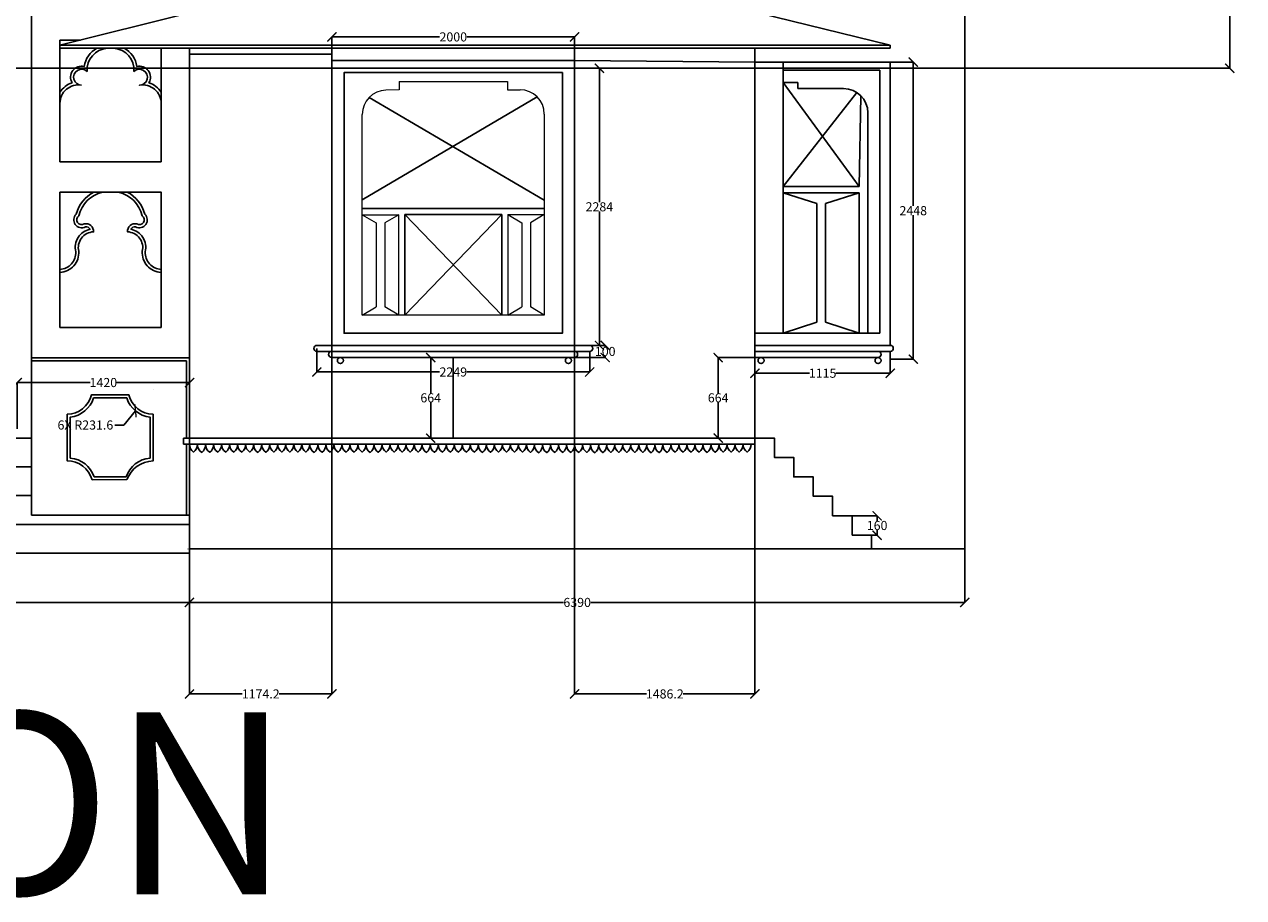
# Model space of a CAD drawing. Units: inches. Extents: x 829 to 33356404, y 1874 to 16983.
# Tile 8 of 9: x 16199 to 26248, y 1874 to 9069. Entities that reach past the tile are written whole.
import ezdxf

# ---------------------------------------------------------------- set-up
doc = ezdxf.new("R2010")
doc.units = ezdxf.units.IN
doc.header["$MEASUREMENT"] = 0
doc.header["$PDMODE"] = 3
for name, color, linetype, lineweight in [('A-ANNO-DIMS', 2, 'Continuous', 18), ('A-ANNO-TEXT', 7, 'Continuous', 25), ('A-ELEV', 7, 'Continuous', 25), ('A-GLAZ', 4, 'Continuous', 18)]:
    doc.layers.add(name, color=color, linetype=linetype, lineweight=lineweight)
doc.styles.get("Standard").update_dxf_attribs({"font": 'arial.ttf'})
doc.dimstyles.get("Standard").update_dxf_attribs({"dimtxt": 75, "dimasz": 75, "dimexe": 0.18, "dimexo": 0.0625, "dimgap": 0.09, "dimtad": 0, "dimtih": 1, "dimtoh": 1, "dimdec": 0, "dimzin": 0, "dimdsep": 46, "dimtxsty": 'Standard', "dimblk": 'ARCHTICK', "dimcen": 0.09, "dimadec": 0, "dimazin": 0, "dimtfac": 1, "dimtdec": 0, "dimtofl": 0, "dimtmove": 0, "dimatfit": 3, "dimfxl": 1, "dimtolj": 1, "dimtzin": 0, "dimarcsym": 0})

# ---------------------------------------------------------------- blocks, each defined once
blk = doc.blocks.new('_ArchTick')
at = {"color": 0, "linetype": 'ByBlock', "const_width": 0.15}
blk.add_lwpolyline([(-0.5, -0.5), (0.5, 0.5)], dxfattribs=at)
blk = doc.blocks.new('*D3')
at = {"layer": 'A-ANNO-DIMS', "color": 0, "lineweight": -2, "transparency": 16777216}
for p, q in [((9560, 4746), (9560, 4306)), ((17560, 4746), (17560, 4306)), ((9560, 4306), (13448, 4306)), ((17560, 4306), (13672, 4306))]:
    blk.add_line(p, q, dxfattribs=at)
at = {"layer": 'Defpoints', "color": 0, "transparency": 16777216}
for p in [(9560, 4746), (17560, 4746), (17560, 4306)]:
    blk.add_point(p, dxfattribs=at)
at = {"layer": 'A-ANNO-DIMS', "color": 0, "lineweight": -2, "transparency": 16777216, "xscale": 75, "yscale": 75, "zscale": 75, "rotation": 180}
blk.add_blockref('_ArchTick', (9560, 4306), dxfattribs=at)
at = {"layer": 'A-ANNO-DIMS', "color": 0, "lineweight": -2, "transparency": 16777216, "xscale": 75, "yscale": 75, "zscale": 75}
blk.add_blockref('_ArchTick', (17560, 4306), dxfattribs=at)
at = {"layer": 'A-ANNO-DIMS', "color": 0, "transparency": 16777216, "insert": (13560, 4306), "char_height": 75, "attachment_point": 5}
blk.add_mtext('\\A1;8000', dxfattribs=at)
blk = doc.blocks.new('*D4')
at = {"layer": 'A-ANNO-DIMS', "color": 0, "lineweight": -2, "transparency": 16777216}
for p, q in [((17560, 4746), (17560, 4306)), ((23950, 4746), (23950, 4306)), ((17560, 4306), (20643, 4306)), ((23950, 4306), (20867, 4306))]:
    blk.add_line(p, q, dxfattribs=at)
at = {"layer": 'Defpoints', "color": 0, "transparency": 16777216}
for p in [(17560, 4746), (23950, 4746), (23950, 4306)]:
    blk.add_point(p, dxfattribs=at)
at = {"layer": 'A-ANNO-DIMS', "color": 0, "lineweight": -2, "transparency": 16777216, "xscale": 75, "yscale": 75, "zscale": 75, "rotation": 180}
blk.add_blockref('_ArchTick', (17560, 4306), dxfattribs=at)
at = {"layer": 'A-ANNO-DIMS', "color": 0, "lineweight": -2, "transparency": 16777216, "xscale": 75, "yscale": 75, "zscale": 75}
blk.add_blockref('_ArchTick', (23950, 4306), dxfattribs=at)
at = {"layer": 'A-ANNO-DIMS', "color": 0, "transparency": 16777216, "insert": (20755, 4306), "char_height": 75, "attachment_point": 5}
blk.add_mtext('\\A1;6390', dxfattribs=at)
blk = doc.blocks.new('*D10')
at = {"layer": 'A-ANNO-DIMS', "color": 0, "lineweight": -2, "transparency": 16777216}
for p, q in [((19734, 6324), (19548, 6324)), ((19548, 6324), (19548, 6031)), ((19548, 5660), (19548, 5954)), ((19734, 5660), (19548, 5660))]:
    blk.add_line(p, q, dxfattribs=at)
at = {"layer": 'Defpoints', "color": 0, "transparency": 16777216}
for p in [(19548, 6324), (19734, 6324), (19734, 5660)]:
    blk.add_point(p, dxfattribs=at)
at = {"layer": 'A-ANNO-DIMS', "color": 0, "lineweight": -2, "transparency": 16777216, "xscale": 75, "yscale": 75, "zscale": 75}
for p, rotation in [((19548, 6324), 90), ((19548, 5660), 270)]:
    blk.add_blockref('_ArchTick', p, dxfattribs=dict(at, rotation=rotation))
at = {"layer": 'A-ANNO-DIMS', "color": 0, "transparency": 16777216, "insert": (19548, 5992), "char_height": 75, "attachment_point": 5}
blk.add_mtext('\\A1;664', dxfattribs=at)
blk = doc.blocks.new('*D11')
at = {"layer": 'A-ANNO-DIMS', "color": 0, "lineweight": -2, "transparency": 16777216}
for p, q in [((22220, 6324), (21916, 6324)), ((21917, 6324), (21917, 6031)), ((21917, 5660), (21917, 5954)), ((22220, 5660), (21916, 5660))]:
    blk.add_line(p, q, dxfattribs=at)
at = {"layer": 'Defpoints', "color": 0, "transparency": 16777216}
for p in [(21917, 6324), (22220, 6324), (22220, 5660)]:
    blk.add_point(p, dxfattribs=at)
at = {"layer": 'A-ANNO-DIMS', "color": 0, "lineweight": -2, "transparency": 16777216, "xscale": 75, "yscale": 75, "zscale": 75}
for p, rotation in [((21917, 6324), 90), ((21917, 5660), 270)]:
    blk.add_blockref('_ArchTick', p, dxfattribs=dict(at, rotation=rotation))
at = {"layer": 'A-ANNO-DIMS', "color": 0, "transparency": 16777216, "insert": (21917, 5992), "char_height": 75, "attachment_point": 5}
blk.add_mtext('\\A1;664', dxfattribs=at)
blk = doc.blocks.new('*D12')
at = {"layer": 'A-ANNO-DIMS', "color": 0, "lineweight": -2, "transparency": 16777216}
for p, q in [((23335, 6374), (23335, 6195)), ((22220, 6310), (22220, 6195)), ((22220, 6195), (22669, 6195)), ((23335, 6195), (22887, 6195))]:
    blk.add_line(p, q, dxfattribs=at)
at = {"layer": 'Defpoints', "color": 0, "transparency": 16777216}
for p in [(23335, 6374), (22220, 6310), (23335, 6195)]:
    blk.add_point(p, dxfattribs=at)
at = {"layer": 'A-ANNO-DIMS', "color": 0, "lineweight": -2, "transparency": 16777216, "xscale": 75, "yscale": 75, "zscale": 75, "rotation": 180}
blk.add_blockref('_ArchTick', (22220, 6195), dxfattribs=at)
at = {"layer": 'A-ANNO-DIMS', "color": 0, "lineweight": -2, "transparency": 16777216, "xscale": 75, "yscale": 75, "zscale": 75}
blk.add_blockref('_ArchTick', (23335, 6195), dxfattribs=at)
at = {"layer": 'A-ANNO-DIMS', "color": 0, "transparency": 16777216, "insert": (22778, 6195), "char_height": 75, "attachment_point": 5}
blk.add_mtext('\\A1;1115', dxfattribs=at)
blk = doc.blocks.new('*D13')
at = {"layer": 'A-ANNO-DIMS', "color": 0, "lineweight": -2, "transparency": 16777216}
for p, q in [((23335, 8758), (23525, 8758)), ((23525, 8758), (23525, 7573)), ((23525, 6310), (23525, 7496)), ((23335, 6310), (23525, 6310))]:
    blk.add_line(p, q, dxfattribs=at)
at = {"layer": 'Defpoints', "color": 0, "transparency": 16777216}
for p in [(23335, 8758), (23525, 8758), (23335, 6310)]:
    blk.add_point(p, dxfattribs=at)
at = {"layer": 'A-ANNO-DIMS', "color": 0, "lineweight": -2, "transparency": 16777216, "xscale": 75, "yscale": 75, "zscale": 75}
for p, rotation in [((23525, 8758), 90), ((23525, 6310), 270)]:
    blk.add_blockref('_ArchTick', p, dxfattribs=dict(at, rotation=rotation))
at = {"layer": 'A-ANNO-DIMS', "color": 0, "transparency": 16777216, "insert": (23525, 7534), "char_height": 75, "attachment_point": 5}
blk.add_mtext('\\A1;2448', dxfattribs=at)
blk = doc.blocks.new('*D18')
at = {"layer": 'A-ANNO-DIMS', "color": 0, "lineweight": -2, "transparency": 16777216}
for p, q in [((16140, 5736), (16140, 6118)), ((16140, 6118), (16741, 6118)), ((17560, 6118), (16958, 6118)), ((17560, 5736), (17560, 6118))]:
    blk.add_line(p, q, dxfattribs=at)
at = {"layer": 'Defpoints', "color": 0, "transparency": 16777216}
for p in [(16140, 6118), (16140, 5735), (17560, 5735)]:
    blk.add_point(p, dxfattribs=at)
at = {"layer": 'A-ANNO-DIMS', "color": 0, "lineweight": -2, "transparency": 16777216, "xscale": 75, "yscale": 75, "zscale": 75, "rotation": 180}
blk.add_blockref('_ArchTick', (16140, 6118), dxfattribs=at)
at = {"layer": 'A-ANNO-DIMS', "color": 0, "lineweight": -2, "transparency": 16777216, "xscale": 75, "yscale": 75, "zscale": 75}
blk.add_blockref('_ArchTick', (17560, 6118), dxfattribs=at)
at = {"layer": 'A-ANNO-DIMS', "color": 0, "transparency": 16777216, "insert": (16850, 6118), "char_height": 75, "attachment_point": 5}
blk.add_mtext('\\A1;1420', dxfattribs=at)
blk = doc.blocks.new('*D29')
at = {"layer": 'A-ANNO-DIMS', "color": 0, "lineweight": -2, "transparency": 16777216}
for p, q in [((18609, 6399), (18609, 6205)), ((20858, 6374), (20858, 6205)), ((18609, 6205), (19621, 6205)), ((20858, 6205), (19847, 6205))]:
    blk.add_line(p, q, dxfattribs=at)
at = {"layer": 'Defpoints', "color": 0, "transparency": 16777216}
for p in [(18609, 6399), (20858, 6374), (20858, 6205)]:
    blk.add_point(p, dxfattribs=at)
at = {"layer": 'A-ANNO-DIMS', "color": 0, "lineweight": -2, "transparency": 16777216, "xscale": 75, "yscale": 75, "zscale": 75, "rotation": 180}
blk.add_blockref('_ArchTick', (18609, 6205), dxfattribs=at)
at = {"layer": 'A-ANNO-DIMS', "color": 0, "lineweight": -2, "transparency": 16777216, "xscale": 75, "yscale": 75, "zscale": 75}
blk.add_blockref('_ArchTick', (20858, 6205), dxfattribs=at)
at = {"layer": 'A-ANNO-DIMS', "color": 0, "transparency": 16777216, "insert": (19734, 6205), "char_height": 75, "attachment_point": 5}
blk.add_mtext('\\A1;2249', dxfattribs=at)
blk = doc.blocks.new('*D30')
at = {"layer": 'A-ANNO-DIMS', "color": 0, "lineweight": -2, "transparency": 16777216}
for p, q in [((20734, 6424), (20986, 6424)), ((20986, 6424), (20986, 6413)), ((20986, 6324), (20986, 6336)), ((20734, 6324), (20986, 6324))]:
    blk.add_line(p, q, dxfattribs=at)
at = {"layer": 'Defpoints', "color": 0, "transparency": 16777216}
for p in [(20734, 6424), (20734, 6324), (20986, 6324)]:
    blk.add_point(p, dxfattribs=at)
at = {"layer": 'A-ANNO-DIMS', "color": 0, "lineweight": -2, "transparency": 16777216, "xscale": 75, "yscale": 75, "zscale": 75}
for p, rotation in [((20986, 6424), 90), ((20986, 6324), 270)]:
    blk.add_blockref('_ArchTick', p, dxfattribs=dict(at, rotation=rotation))
at = {"layer": 'A-ANNO-DIMS', "color": 0, "transparency": 16777216, "insert": (20986, 6374), "char_height": 75, "attachment_point": 5}
blk.add_mtext('\\A1;100', dxfattribs=at)
blk = doc.blocks.new('*D31')
at = {"layer": 'A-ANNO-DIMS', "color": 0, "lineweight": -2, "transparency": 16777216}
for p, q in [((20734, 8708), (20938, 8708)), ((20938, 8708), (20938, 7605)), ((20938, 6424), (20938, 7528)), ((20734, 6424), (20938, 6424))]:
    blk.add_line(p, q, dxfattribs=at)
at = {"layer": 'Defpoints', "color": 0, "transparency": 16777216}
for p in [(20734, 8708), (20734, 6424), (20938, 6424)]:
    blk.add_point(p, dxfattribs=at)
at = {"layer": 'A-ANNO-DIMS', "color": 0, "lineweight": -2, "transparency": 16777216, "xscale": 75, "yscale": 75, "zscale": 75}
for p, rotation in [((20938, 8708), 90), ((20938, 6424), 270)]:
    blk.add_blockref('_ArchTick', p, dxfattribs=dict(at, rotation=rotation))
at = {"layer": 'A-ANNO-DIMS', "color": 0, "transparency": 16777216, "insert": (20938, 7566), "char_height": 75, "attachment_point": 5}
blk.add_mtext('\\A1;2284', dxfattribs=at)
blk = doc.blocks.new('*D32')
at = {"layer": 'A-ANNO-DIMS', "color": 0, "lineweight": -2, "transparency": 16777216}
for p, q in [((23020, 5020), (23227, 5020)), ((23227, 5020), (23227, 4979)), ((23020, 4860), (23227, 4860)), ((23227, 4860), (23227, 4902))]:
    blk.add_line(p, q, dxfattribs=at)
at = {"layer": 'Defpoints', "color": 0, "transparency": 16777216}
for p in [(23020, 5020), (23227, 5020), (23020, 4860)]:
    blk.add_point(p, dxfattribs=at)
at = {"layer": 'A-ANNO-DIMS', "color": 0, "lineweight": -2, "transparency": 16777216, "xscale": 75, "yscale": 75, "zscale": 75}
for p, rotation in [((23227, 5020), 90), ((23227, 4860), 270)]:
    blk.add_blockref('_ArchTick', p, dxfattribs=dict(at, rotation=rotation))
at = {"layer": 'A-ANNO-DIMS', "color": 0, "transparency": 16777216, "insert": (23227, 4940), "char_height": 75, "attachment_point": 5}
blk.add_mtext('\\A1;160', dxfattribs=at)
blk = doc.blocks.new('*D64')
at = {"layer": 'A-ANNO-DIMS', "color": 0, "lineweight": -2, "transparency": 16777216}
for p, q in [((18734, 8773), (18734, 8967)), ((18734, 8966), (19621, 8966)), ((20734, 8966), (19847, 8966)), ((20734, 8773), (20734, 8967))]:
    blk.add_line(p, q, dxfattribs=at)
at = {"layer": 'Defpoints', "color": 0, "transparency": 16777216}
for p in [(20734, 8966), (18734, 8772), (20734, 8772)]:
    blk.add_point(p, dxfattribs=at)
at = {"layer": 'A-ANNO-DIMS', "color": 0, "lineweight": -2, "transparency": 16777216, "xscale": 75, "yscale": 75, "zscale": 75, "rotation": 180}
blk.add_blockref('_ArchTick', (18734, 8966), dxfattribs=at)
at = {"layer": 'A-ANNO-DIMS', "color": 0, "lineweight": -2, "transparency": 16777216, "xscale": 75, "yscale": 75, "zscale": 75}
blk.add_blockref('_ArchTick', (20734, 8966), dxfattribs=at)
at = {"layer": 'A-ANNO-DIMS', "color": 0, "transparency": 16777216, "insert": (19734, 8966), "char_height": 75, "attachment_point": 5}
blk.add_mtext('\\A1;2000', dxfattribs=at)
blk = doc.blocks.new('WIN-ARCHED')
for p, q in [((304, 1923), (1196, 1923)), ((304, 1923), (304, 1856)), ((1196, 1923), (1196, 1856)), ((304, 1856), (195, 1853)), ((1196, 1856), (1300, 1856)), ((0, 0), (0, 1653)), ((1500, 1656), (1500, 0)), ((0, 827), (300, 827)), ((0, 827), (115, 759)), ((300, 827), (185, 759)), ((300, 0), (300, 827)), ((1200, 828), (1200, 0)), ((1200, 828), (1500, 828)), ((1200, 828), (1315, 760)), ((1500, 828), (1385, 760)), ((115, 759), (115, 68)), ((185, 759), (185, 68)), ((1315, 760), (1315, 68)), ((1385, 760), (1385, 68)), ((0, 0), (115, 68)), ((1500, 0), (0, 0)), ((300, 0), (185, 68)), ((1200, 0), (1315, 68)), ((1500, 0), (1385, 68))]:
    blk.add_line(p, q)
for centre, start, end in [((200, 1653), 91.5254, 180), ((1300, 1656), 0, 90)]:
    blk.add_arc(centre, 200, start, end)
blk = doc.blocks.new('*D88')
at = {"layer": 'A-ANNO-DIMS', "color": 0, "lineweight": -2, "transparency": 16777216}
for p, q in [((18734, 6424), (18734, 3551)), ((17560, 6321), (17560, 3551)), ((17560, 3552), (17995, 3552)), ((18734, 3552), (18299, 3552))]:
    blk.add_line(p, q, dxfattribs=at)
at = {"layer": 'Defpoints', "color": 0, "transparency": 16777216}
for p in [(18734, 6424), (17560, 6321), (18734, 3552)]:
    blk.add_point(p, dxfattribs=at)
at = {"layer": 'A-ANNO-DIMS', "color": 0, "lineweight": -2, "transparency": 16777216, "xscale": 75, "yscale": 75, "zscale": 75, "rotation": 180}
blk.add_blockref('_ArchTick', (17560, 3552), dxfattribs=at)
at = {"layer": 'A-ANNO-DIMS', "color": 0, "lineweight": -2, "transparency": 16777216, "xscale": 75, "yscale": 75, "zscale": 75}
blk.add_blockref('_ArchTick', (18734, 3552), dxfattribs=at)
at = {"layer": 'A-ANNO-DIMS', "color": 0, "transparency": 16777216, "insert": (18147, 3552), "char_height": 75, "attachment_point": 5}
blk.add_mtext('\\A1;1174.2', dxfattribs=at)
blk = doc.blocks.new('*D89')
at = {"layer": 'A-ANNO-DIMS', "color": 0, "lineweight": -2, "transparency": 16777216}
for p, q in [((20734, 6424), (20734, 3551)), ((22220, 6324), (22220, 3551)), ((20734, 3552), (21325, 3552)), ((22220, 3552), (21629, 3552))]:
    blk.add_line(p, q, dxfattribs=at)
at = {"layer": 'Defpoints', "color": 0, "transparency": 16777216}
for p in [(20734, 6424), (22220, 6324), (22220, 3552)]:
    blk.add_point(p, dxfattribs=at)
at = {"layer": 'A-ANNO-DIMS', "color": 0, "lineweight": -2, "transparency": 16777216, "xscale": 75, "yscale": 75, "zscale": 75, "rotation": 180}
blk.add_blockref('_ArchTick', (20734, 3552), dxfattribs=at)
at = {"layer": 'A-ANNO-DIMS', "color": 0, "lineweight": -2, "transparency": 16777216, "xscale": 75, "yscale": 75, "zscale": 75}
blk.add_blockref('_ArchTick', (22220, 3552), dxfattribs=at)
at = {"layer": 'A-ANNO-DIMS', "color": 0, "transparency": 16777216, "insert": (21477, 3552), "char_height": 75, "attachment_point": 5}
blk.add_mtext('\\A1;1486.2', dxfattribs=at)
blk = doc.blocks.new('*D91')
at = {"layer": 'A-ANNO-DIMS', "color": 0, "lineweight": -2, "transparency": 16777216}
for p, q in [((11082, 9925), (26134, 9925)), ((26134, 9925), (26134, 9355)), ((26134, 8708), (26134, 9279)), ((11082, 8708), (26134, 8708))]:
    blk.add_line(p, q, dxfattribs=at)
at = {"layer": 'Defpoints', "color": 0, "transparency": 16777216}
for p in [(11082, 9925), (11082, 8708), (26134, 8708)]:
    blk.add_point(p, dxfattribs=at)
at = {"layer": 'A-ANNO-DIMS', "color": 0, "lineweight": -2, "transparency": 16777216, "xscale": 75, "yscale": 75, "zscale": 75}
for p, rotation in [((26134, 9925), 90), ((26134, 8708), 270)]:
    blk.add_blockref('_ArchTick', p, dxfattribs=dict(at, rotation=rotation))
at = {"layer": 'A-ANNO-DIMS', "color": 0, "transparency": 16777216, "insert": (26134, 9317), "char_height": 75, "attachment_point": 5}
blk.add_mtext('\\A1;1217', dxfattribs=at)
blk = doc.blocks.new('*D137')
at = {"layer": 'A-ANNO-DIMS', "color": 0, "lineweight": -2, "transparency": 16777216}
for p, q in [((17262, 6063), (17263, 6063)), ((17262, 6063), (17262, 6063)), ((17020, 5768), (17115, 5884)), ((16945, 5768), (17020, 5768))]:
    blk.add_line(p, q, dxfattribs=at)
at = {"layer": 'Defpoints', "color": 0, "transparency": 16777216}
for p in [(17262, 6063), (17115, 5884)]:
    blk.add_point(p, dxfattribs=at)
at = {"layer": 'A-ANNO-DIMS', "color": 0, "lineweight": -2, "transparency": 16777216, "xscale": 75, "yscale": 75, "zscale": 75, "rotation": 50.57670159056939}
blk.add_blockref('_ArchTick', (17115, 5884), dxfattribs=at)
at = {"layer": 'A-ANNO-DIMS', "color": 0, "transparency": 16777216, "insert": (16702, 5768), "char_height": 75, "attachment_point": 5}
blk.add_mtext('\\A1;6X R231.6', dxfattribs=at)

msp = doc.modelspace()

# ---------------------------------------------------------------- linework, layer by layer
at = {"layer": 'A-ELEV'}
for p, q in [((23949.778, 4746.468), (23949.778, 13204.032)), ((16258.701, 12127.212), (16258.701, 5024.468)), ((17559.22, 9165.468), (16492.651, 8897.385)), ((23335.316, 8897.468), (22247.13, 9165.468)), ((16492.651, 8897.385), (16492.651, 8940.247)), ((16492.651, 8940.247), (16662.702, 8940.128)), ((23335.316, 8897.468), (16492.651, 8897.468)), ((23335.316, 8872.468), (16492.651, 8872.468)), ((17559.778, 5660.468), (17559.778, 8872.468)), ((22220.173, 8872.468), (22220.173, 5610.468)), ((23335.316, 8897.468), (23335.316, 8872.468)), ((18733.997, 8824.567), (17559.778, 8824.567)), ((18733.997, 6424.468), (18733.997, 8772.468)), ((18733.997, 8772.468), (20733.997, 8772.468)), ((20733.997, 8772.468), (20733.997, 6424.468)), ((20733.997, 8772.468), (22220.46, 8758.159)), ((22220.173, 8758.159), (23335.173, 8758.159)), ((22453.679, 8758.159), (22453.679, 6524.468)), ((23335.173, 8758.159), (23335.173, 6424.468)), ((22220.173, 8708.159), (20733.997, 8708.249)), ((22453.679, 8692.423), (23250.644, 8692.423)), ((23250.644, 8692.423), (23250.644, 6524.468)), ((22453.679, 8590.899), (22453.679, 8590.899)), ((22453.679, 8590.899), (22574.492, 8590.899)), ((23079.068, 7732.894), (22453.679, 8590.899)), ((22574.492, 8590.899), (22574.492, 8540.137)), ((18983.997, 7623.901), (20425.418, 8471.984)), ((19040.705, 8467.25), (20483.997, 7621.325)), ((22453.679, 7732.894), (23060.564, 8507.223)), ((22574.492, 8540.137), (22950.644, 8540.137)), ((23079.068, 7732.894), (23092.065, 8481.558)), ((23150.644, 8340.137), (23150.644, 6524.468)), ((22453.679, 7732.894), (23079.068, 7732.894)), ((22453.679, 7682.132), (23079.068, 7682.132)), ((22453.679, 7682.132), (22730.84, 7592.059)), ((23079.068, 7682.132), (22801.907, 7592.059)), ((23079.068, 7682.132), (23079.068, 6524.468)), ((18983.949, 7551.096), (20483.949, 7552.516)), ((20233.997, 7552.326), (20233.997, 7552.279)), ((22730.84, 7592.059), (22730.84, 6614.542)), ((22801.907, 7592.059), (22801.907, 6614.542)), ((19098.997, 7501.214), (19098.997, 7501.187)), ((19333.997, 6674.468), (19333.997, 7501.38)), ((19333.997, 7501.38), (20133.997, 7501.38)), ((20133.997, 7501.38), (19333.997, 6674.468)), ((19333.997, 7501.332), (20133.997, 6674.468)), ((20133.997, 7502.232), (20133.997, 6674.468)), ((20298.997, 7502.397), (20298.997, 7502.37)), ((22453.679, 6524.468), (22730.84, 6614.542)), ((23079.068, 6524.468), (22801.907, 6614.542)), ((23250.644, 6524.468), (22220.173, 6524.468)), ((22475.769, 6524.468), (23151.92, 6524.468)), ((18609.497, 6424.468), (18733.997, 6424.468)), ((18609.497, 6374.468), (20858.497, 6374.468)), ((20733.997, 6424.468), (18733.997, 6424.468)), ((20858.497, 6424.468), (20733.997, 6424.468)), ((23335.173, 6424.468), (22220.173, 6424.468)), ((23335.173, 6374.468), (22220.173, 6374.468)), ((16258.692, 6296.468), (17534.778, 6296.307)), ((16258.695, 6321.468), (17559.778, 6321.304)), ((17534.778, 6296.307), (17534.778, 5660.468)), ((18731.471, 6324.468), (20733.997, 6324.468)), ((19733.997, 5660.468), (19733.997, 6324.468)), ((23235.173, 6324.468), (22220.173, 6324.468)), ((10860.89, 5660.468), (16258.701, 5660.468)), ((17509.778, 5660.468), (22220.173, 5660.468)), ((17509.778, 5660.468), (17509.778, 5610.468)), ((17509.778, 5610.468), (22220.173, 5610.468)), ((17534.778, 5610.468), (17534.778, 5024.468)), ((17559.778, 4746.468), (17559.778, 5610.468)), ((16258.701, 5423.468), (10979.778, 5423.468)), ((16258.701, 5186.468), (10979.778, 5186.468)), ((16258.579, 5024.468), (17559.778, 5024.468)), ((9559.778, 4949.468), (17559.778, 4949.468)), ((23020.173, 4860.468), (23180.173, 4860.468)), ((23180.173, 4860.468), (23180.173, 4746.468)), ((17549.891, 4746.468), (17549.891, 4746.304)), ((17559.778, 4746.468), (23949.778, 4746.468)), ((17668.891, 4746.468), (17668.891, 4746.289)), ((17768.891, 4746.468), (17768.891, 4746.276)), ((17843.891, 4746.468), (17843.891, 4746.267)), ((23949.778, 4746.468), (23789.778, 4746.468)), ((9559.778, 4711.528), (17559.778, 4711.528))]:
    msp.add_line(p, q, dxfattribs=at)
for points in [[(17325.828, 8872.468), (17325.828, 7937.261), (16492.651, 7937.261), (16492.651, 8897.385)], [(23020.173, 4860.468), (23020.173, 5020.468), (22860.173, 5020.468), (22860.173, 5180.468), (22700.173, 5180.468), (22700.173, 5340.468), (22540.173, 5340.468), (22540.173, 5500.468), (22380.173, 5500.468), (22380.173, 5660.468), (22220.173, 5660.468)], [(17037.537, 5340.542), (16773.358, 5340.542)], [(17043.578, 5317.852), (16756.777, 5317.468)]]:
    msp.add_lwpolyline(points, dxfattribs=at)
for points in [[(16592.612, 8587.794, -0.665289385), (16692.599, 8722.287, -0.23532644), (16796.033, 8872.468, -0.23532644)], [(16670.776, 8568.249, -1.473007826), (16715.947, 8682.012, -0.409891223), (16880.813, 8872.468)], [(16937.666, 8872.468, -0.409891223), (17102.532, 8682.012, -1.473007826), (17147.703, 8568.249, -0.471652219), (17325.828, 8416.104)], [(17022.446, 8872.468, -0.23532644), (17125.88, 8722.287, -0.665289385), (17225.867, 8587.794, -0.185809429), (17325.828, 8509.437, -0.185809429)], [(16491.331, 7049.962, 0.418566918), (16622.283, 7195.519, -0.418044948), (16740.242, 7381.328, 0.322328475), (16702.182, 7401.223, -0.879192404), (16626.718, 7506.037, -0.211560791), (16771.599, 7687.262, -0.211560791)], [(16492.464, 7024.987), (16492.464, 7024.987, 0.422659313), (16647.086, 7199.277, -0.477145618), (16768.947, 7359.767, 0.509446731), (16693.183, 7424.938, -0.995850689), (16648.97, 7491.881, -0.284123673), (16842.407, 7687.262)], [(17325.642, 7024.987), (17325.642, 7024.987, -0.422659313), (17171.02, 7199.277, 0.477145618), (17049.159, 7359.767, -0.509446731), (17124.923, 7424.938, 0.995850689), (17169.136, 7491.881, 0.284123673), (16975.699, 7687.262)], [(17326.775, 7049.962, -0.418566918), (17195.823, 7195.519, 0.418044948), (17077.864, 7381.328, -0.322328475), (17115.924, 7401.223, 0.879192404), (17191.388, 7506.037, 0.211560791), (17046.507, 7687.262, 0.211560791)], [(16756.777, 5317.468, 0.341381101), (16552.757, 5471.984), (16552.757, 5856.29, 0.344613803), (16751.006, 6015.968), (17061.229, 6015.968, 0.344613803), (17259.478, 5856.29), (17259.478, 5471.984, 0.304717221), (17043.578, 5317.852, 0.324302379)], [(16773.358, 5340.542, 0.298822494), (16577.757, 5495.944), (16577.757, 5832.963, 0.291379911), (16769.956, 5990.968), (17042.279, 5990.968, 0.291379911), (17234.478, 5832.963), (17234.478, 5495.944, 0.29428256), (17037.527, 5340.513)], [(17559.778, 5610.468, 0.267810975), (17594.235, 5544.592, 0.244698443), (17625.867, 5610.468, 0.244698443)], [(17625.909, 5610.468, 0.275125954), (17660.366, 5542.037, 0.251670242), (17691.998, 5610.468, 0.244698443)], [(17692.07, 5609.062, 0.267810975), (17726.527, 5543.186, 0.244698443), (17758.16, 5609.062, 0.244698443)], [(17758.26, 5610.468, 0.267810975), (17792.717, 5544.592, 0.244698443), (17824.349, 5610.468, 0.244698443)], [(17824.26, 5610.463, 0.267810975), (17858.718, 5544.587, 0.244698443), (17890.35, 5610.463, 0.244698443)], [(17890.453, 5610.468, 0.267810975), (17924.91, 5544.592, 0.244698443), (17956.542, 5610.468, 0.244698443)], [(17956.542, 5610.468, 0.267810975), (17990.999, 5544.592, 0.244698443), (18022.632, 5610.468, 0.244698443)], [(18022.695, 5610.468, 0.267810975), (18057.153, 5544.592, 0.244698443), (18088.785, 5610.468, 0.244698443)], [(18088.826, 5610.468, 0.275125954), (18123.283, 5542.037, 0.251670242), (18154.915, 5610.468, 0.244698443)], [(18154.987, 5609.062, 0.267810975), (18189.445, 5543.186, 0.244698443), (18221.077, 5609.062, 0.244698443)], [(18221.177, 5610.468, 0.267810975), (18255.634, 5544.592, 0.244698443), (18287.266, 5610.468, 0.244698443)], [(18287.177, 5610.463, 0.267810975), (18321.635, 5544.587, 0.244698443), (18353.267, 5610.463, 0.244698443)], [(18353.37, 5610.468, 0.267810975), (18387.827, 5544.592, 0.244698443), (18419.459, 5610.468, 0.244698443)], [(18419.459, 5610.468, 0.267810975), (18453.917, 5544.592, 0.244698443), (18485.549, 5610.468, 0.244698443)], [(18485.549, 5610.468, 0.267810975), (18520.006, 5544.592, 0.244698443), (18551.638, 5610.468, 0.244698443)], [(18551.679, 5610.468, 0.275125954), (18586.137, 5542.037, 0.251670242), (18617.769, 5610.468, 0.244698443)], [(18617.841, 5609.062, 0.267810975), (18652.298, 5543.186, 0.244698443), (18683.93, 5609.062, 0.244698443)], [(18684.03, 5610.468, 0.267810975), (18718.487, 5544.592, 0.244698443), (18750.12, 5610.468, 0.244698443)], [(18750.031, 5610.463, 0.267810975), (18784.488, 5544.587, 0.244698443), (18816.12, 5610.463, 0.244698443)], [(18816.224, 5610.468, 0.267810975), (18850.681, 5544.592, 0.244698443), (18882.313, 5610.468, 0.244698443)], [(18882.313, 5610.468, 0.267810975), (18916.77, 5544.592, 0.244698443), (18948.402, 5610.468, 0.244698443)], [(18948.466, 5610.468, 0.267810975), (18982.923, 5544.592, 0.244698443), (19014.555, 5610.468, 0.244698443)], [(19014.596, 5610.468, 0.275125954), (19049.054, 5542.037, 0.251670242), (19080.686, 5610.468, 0.244698443)], [(19080.758, 5609.062, 0.267810975), (19115.215, 5543.186, 0.244698443), (19146.847, 5609.062, 0.244698443)], [(19146.947, 5610.468, 0.267810975), (19181.405, 5544.592, 0.244698443), (19213.037, 5610.468, 0.244698443)], [(19212.948, 5610.463, 0.267810975), (19247.405, 5544.587, 0.244698443), (19279.037, 5610.463, 0.244698443)], [(19279.141, 5610.468, 0.267810975), (19313.598, 5544.592, 0.244698443), (19345.23, 5610.468, 0.244698443)], [(19345.23, 5610.468, 0.267810975), (19379.687, 5544.592, 0.244698443), (19411.319, 5610.468, 0.244698443)], [(19411.319, 5610.468, 0.267810975), (19445.777, 5544.592, 0.244698443), (19477.409, 5610.468, 0.244698443)], [(19477.45, 5610.468, 0.275125954), (19511.907, 5542.037, 0.251670242), (19543.539, 5610.468, 0.244698443)], [(19543.611, 5609.062, 0.267810975), (19578.069, 5543.186, 0.244698443), (19609.701, 5609.062, 0.244698443)], [(19609.801, 5610.468, 0.267810975), (19644.258, 5544.592, 0.244698443), (19675.89, 5610.468, 0.244698443)], [(19675.801, 5610.463, 0.267810975), (19710.259, 5544.587, 0.244698443), (19741.891, 5610.463, 0.244698443)], [(19741.994, 5610.468, 0.267810975), (19776.451, 5544.592, 0.244698443), (19808.083, 5610.468, 0.244698443)], [(19808.083, 5610.468, 0.267810975), (19842.541, 5544.592, 0.244698443), (19874.173, 5610.468, 0.244698443)], [(19874.236, 5610.468, 0.267810975), (19908.694, 5544.592, 0.244698443), (19940.326, 5610.468, 0.244698443)], [(19940.367, 5610.468, 0.275125954), (19974.824, 5542.037, 0.251670242), (20006.456, 5610.468, 0.244698443)], [(20006.529, 5609.062, 0.267810975), (20040.986, 5543.186, 0.244698443), (20072.618, 5609.062, 0.244698443)], [(20072.718, 5610.468, 0.267810975), (20107.175, 5544.592, 0.244698443), (20138.807, 5610.468, 0.244698443)], [(20138.719, 5610.463, 0.267810975), (20173.176, 5544.587, 0.244698443), (20204.808, 5610.463, 0.244698443)], [(20204.911, 5610.468, 0.267810975), (20239.368, 5544.592, 0.244698443), (20271.001, 5610.468, 0.244698443)], [(20271.001, 5610.468, 0.267810975), (20305.458, 5544.592, 0.244698443), (20337.09, 5610.468, 0.244698443)], [(20337.131, 5607.838, 0.267810975), (20371.588, 5541.962, 0.244698443), (20403.22, 5607.838, 0.244698443)], [(20403.262, 5607.838, 0.275125954), (20437.719, 5539.406, 0.251670242), (20469.351, 5607.838, 0.244698443)], [(20469.423, 5606.431, 0.267810975), (20503.88, 5540.555, 0.244698443), (20535.512, 5606.431, 0.244698443)], [(20535.613, 5607.838, 0.267810975), (20570.07, 5541.962, 0.244698443), (20601.702, 5607.838, 0.244698443)], [(20601.613, 5607.832, 0.267810975), (20636.07, 5541.956, 0.244698443), (20667.703, 5607.832, 0.244698443)], [(20667.806, 5607.838, 0.267810975), (20702.263, 5541.962, 0.244698443), (20733.895, 5607.838, 0.244698443)], [(20733.895, 5607.838, 0.267810975), (20768.352, 5541.962, 0.244698443), (20799.984, 5607.838, 0.244698443)], [(20800.048, 5607.838, 0.267810975), (20834.506, 5541.962, 0.244698443), (20866.138, 5607.838, 0.244698443)], [(20866.179, 5607.838, 0.275125954), (20900.636, 5539.406, 0.251670242), (20932.268, 5607.838, 0.244698443)], [(20932.34, 5606.431, 0.267810975), (20966.798, 5540.555, 0.244698443), (20998.43, 5606.431, 0.244698443)], [(20998.53, 5607.838, 0.267810975), (21032.987, 5541.962, 0.244698443), (21064.619, 5607.838, 0.244698443)], [(21064.53, 5607.832, 0.267810975), (21098.988, 5541.956, 0.244698443), (21130.62, 5607.832, 0.244698443)], [(21130.723, 5607.838, 0.267810975), (21165.18, 5541.962, 0.244698443), (21196.812, 5607.838, 0.244698443)], [(21196.812, 5607.838, 0.267810975), (21231.27, 5541.962, 0.244698443), (21262.902, 5607.838, 0.244698443)], [(21262.902, 5607.838, 0.267810975), (21297.359, 5541.962, 0.244698443), (21328.991, 5607.838, 0.244698443)], [(21329.032, 5607.838, 0.275125954), (21363.489, 5539.406, 0.251670242), (21395.122, 5607.838, 0.244698443)], [(21395.194, 5606.431, 0.267810975), (21429.651, 5540.555, 0.244698443), (21461.283, 5606.431, 0.244698443)], [(21461.383, 5607.838, 0.267810975), (21495.84, 5541.962, 0.244698443), (21527.472, 5607.838, 0.244698443)], [(21527.384, 5610.463, 0.267810975), (21561.841, 5544.587, 0.244698443), (21593.473, 5610.463, 0.244698443)], [(21593.576, 5610.468, 0.267810975), (21628.034, 5544.592, 0.244698443), (21659.666, 5610.468, 0.244698443)], [(21659.666, 5610.468, 0.267810975), (21694.123, 5544.592, 0.244698443), (21725.755, 5610.468, 0.244698443)], [(21725.819, 5610.468, 0.267810975), (21760.276, 5544.592, 0.244698443), (21791.908, 5610.468, 0.244698443)], [(21791.949, 5610.468, 0.275125954), (21826.407, 5542.037, 0.251670242), (21858.039, 5610.468, 0.244698443)], [(21858.111, 5609.062, 0.267810975), (21892.568, 5543.186, 0.244698443), (21924.2, 5609.062, 0.244698443)], [(21924.3, 5610.468, 0.267810975), (21958.758, 5544.592, 0.244698443), (21990.39, 5610.468, 0.244698443)], [(21990.301, 5610.463, 0.267810975), (22024.758, 5544.587, 0.244698443), (22056.39, 5610.463, 0.244698443)], [(22056.494, 5610.468, 0.267810975), (22090.951, 5544.592, 0.244698443), (22122.583, 5610.468, 0.244698443)], [(22122.583, 5610.468, 0.267810975), (22157.04, 5544.592, 0.244698443), (22188.672, 5610.468, 0.244698443)]]:
    msp.add_lwpolyline(points, format="xyb", dxfattribs=at)
for points in [[(20633.997, 8672.468), (20633.997, 6524.468), (18833.997, 6524.468), (18833.997, 8672.468)], [(16492.464, 7687.262), (17325.642, 7687.262), (17325.642, 6572.436), (16492.464, 6572.436)]]:
    msp.add_lwpolyline(points, close=True, dxfattribs=at)
for centre in [(18803.475, 6299.468), (20682.47, 6299.468), (22270.88, 6299.468), (23235.265, 6299.468)]:
    msp.add_circle(centre, 25, dxfattribs=at)
for centre, radius, start, end in [((16644.418, 8418.764), 151.79, 80, 181.0040496), ((16644.418, 8418.764), 176.79, 107.0396403, 149.1438554), ((22950.644, 8340.137), 200, 0, 90), ((18609.497, 6399.468), 25, 90, 270), ((18731.471, 6349.468), 25, 90, 270), ((20733.997, 6349.468), 25, 270, 90), ((20858.497, 6399.468), 25, 270, 90), ((23235.173, 6349.468), 25, 270, 90), ((23335.173, 6399.468), 25, 270, 90)]:
    msp.add_arc(centre, radius, start, end, dxfattribs=at)

# ---------------------------------------------------------------- block references
at = {"layer": 'A-GLAZ'}
msp.add_blockref('WIN-ARCHED', (18983.997, 6674.232), dxfattribs=at)

# ---------------------------------------------------------------- texts
at = {"layer": 'A-ANNO-TEXT'}
msp.add_text('ELEVATION', height=1500, dxfattribs=at).set_placement((7631.721, 1900.346))

# ---------------------------------------------------------------- dimensions: what is measured, and where the dimension line sits
at = {"layer": 'A-ANNO-DIMS'}
for base, p1, p2, override, picture, middle in [((26133.929, 8708.468), (11081.778, 9925.468), (11081.778, 8708.468), {"dimdec": 0, "dimlfac": 1, "dimrnd": 0, "dimzin": 0, "dimdsep": 46, "dimlunit": 2}, '*D91', (26133.929, 9316.968)), ((20937.969, 6424.468), (20733.997, 8708.249), (20733.997, 6424.468), {"dimclrd": 0, "dimclre": 0, "dimclrt": 0}, '*D31', (20937.969, 7566.358)), ((20985.508, 6324.468), (20733.997, 6424.468), (20733.997, 6324.468), {"dimclrd": 0, "dimclre": 0, "dimclrt": 0}, '*D30', (20985.508, 6374.468)), ((21916.508, 6324.468), (22220.173, 5660.468), (22220.173, 6324.468), {"dimclrd": 0, "dimclre": 0, "dimclrt": 0}, '*D11', (21916.508, 5992.468)), ((23226.559, 5020.468), (23020.173, 4860.468), (23020.173, 5020.468), {"dimclrd": 0, "dimclre": 0, "dimclrt": 0}, '*D32', (23226.559, 4940.468))]:
    dim = msp.add_linear_dim(base=base, p1=p1, p2=p2, angle=90, dimstyle='Standard', override=override, dxfattribs=at)
    dim.commit()
    dim.dimension.update_dxf_attribs({"geometry": picture, "text_midpoint": middle})
for base, p1, p2, override, picture, middle in [((20733.997, 8966.448), (18733.997, 8772.468), (20733.997, 8772.468), {"dimclrd": 0, "dimclre": 0, "dimclrt": 0}, '*D64', (19733.997, 8966.448)), ((18733.997, 3551.528), (17559.778, 6321.304), (18733.997, 6424.468), {"dimdec": 1, "dimlfac": 1, "dimrnd": 0, "dimzin": 0, "dimdsep": 46, "dimlunit": 2}, '*D88', (18146.887, 3551.528)), ((20858.497, 6205.007), (18609.497, 6399.468), (20858.497, 6374.468), {"dimclrd": 0, "dimclre": 0, "dimclrt": 0}, '*D29', (19733.997, 6205.007)), ((22220.173, 3551.528), (20733.997, 6424.468), (22220.173, 6324.468), {"dimdec": 1, "dimlfac": 1, "dimrnd": 0, "dimzin": 0, "dimdsep": 46, "dimlunit": 2}, '*D89', (21477.085, 3551.528)), ((16139.685, 6118.028), (17559.778, 5735.468), (16139.685, 5735.461), {"dimclrd": 0, "dimclre": 0, "dimclrt": 0}, '*D18', (16849.732, 6118.028)), ((17559.778, 4306.306), (9559.778, 4746.468), (17559.778, 4746.468), {"dimclrd": 0, "dimclre": 0, "dimclrt": 0}, '*D3', (13559.778, 4306.306)), ((23949.778, 4306.306), (17559.778, 4746.468), (23949.778, 4746.468), {"dimclrd": 0, "dimclre": 0, "dimclrt": 0}, '*D4', (20754.778, 4306.306))]:
    dim = msp.add_linear_dim(base=base, p1=p1, p2=p2, dimstyle='Standard', override=override, dxfattribs=at)
    dim.commit()
    dim.dimension.update_dxf_attribs({"geometry": picture, "text_midpoint": middle})
for base, p1, p2, picture, middle in [((23525.15, 8758.159), (23335.173, 6310.159), (23335.173, 8758.159), '*D13', (23525.15, 7534.159)), ((19548.218, 6324.468), (19733.997, 5660.468), (19733.997, 6324.468), '*D10', (19548.218, 5992.468))]:
    dim = msp.add_linear_dim(base=base, p1=p1, p2=p2, angle=90, dimstyle='Standard', override={"dimclrd": 0, "dimclre": 0, "dimclrt": 0}, dxfattribs=at)
    dim.commit()
    dim.dimension.update_dxf_attribs({"geometry": picture, "text_midpoint": middle, "dimtype": 160})
dim = msp.add_linear_dim(base=(23335.173, 6195.22), p1=(22220.173, 6309.723), p2=(23335.173, 6374.468), dimstyle='Standard', override={"dimclrd": 0, "dimclre": 0, "dimclrt": 0}, dxfattribs=at)
dim.commit()
dim.dimension.update_dxf_attribs({"geometry": '*D12', "text_midpoint": (22777.673, 6195.22), "dimtype": 160})
dim = msp.add_radius_dim(center=(17262.435, 6062.869), mpoint=(17115.359, 5883.964), text='6X <>', dimstyle='Standard', override={"dimdec": 1, "dimlfac": 1, "dimrnd": 0, "dimzin": 0, "dimdsep": 46, "dimlunit": 2}, dxfattribs=at)
dim.commit()
dim.dimension.update_dxf_attribs({"geometry": '*D137', "text_midpoint": (16701.825, 5768.093)})

doc.saveas('drawing.dxf')
